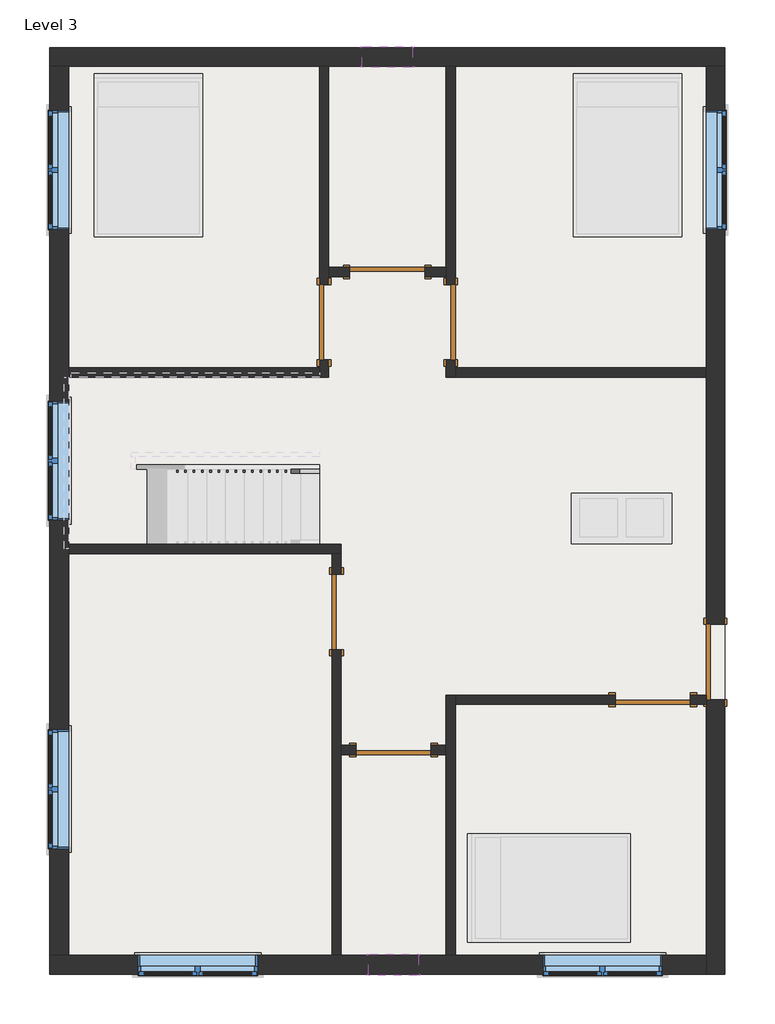
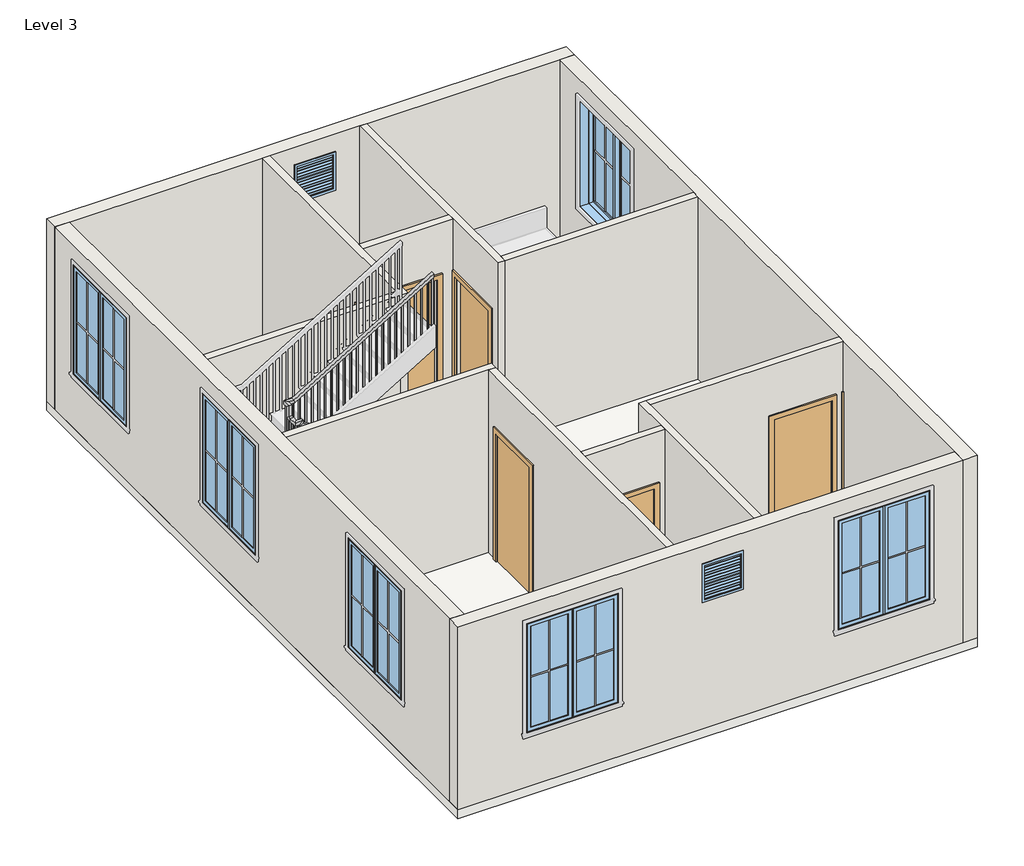
# One storey, part 1 of 2: 14 walls, 8 windows, 7 doors, 1 railing, 1 slab.
"""IFC4 building model written with IfcOpenShell, lengths in millimetres."""

from ifc_helpers import new_model, si_unit, frame, origin, place, context, project, spatial, polyline, outline, extrude, faceted_brep, transform, mapped, element, save
from components import door_305aa2a5, door_e5f9f3c4, door_0ca8825f, window_9ac97e1a, window_f2d8fef0

model = new_model("IFC4")

# Units and contexts
model_context = context("Model", 3, world=origin())
ifc_project = project(units=[si_unit("LENGTHUNIT", "METRE", prefix="MILLI")], contexts=[model_context])

# Site, building, storey
site = spatial("IfcSite", under=ifc_project)
building = spatial("IfcBuilding", under=site)
storey = spatial("IfcBuildingStorey", under=building, Name="Level 3", Elevation=3200.4)

# Doors
placement = place(None, origin())
door_shape = door_305aa2a5(model_context)
element("IfcDoor", 1, ObjectType="Single-Flush : 36\" x 84\"", at=placement, inside=storey, context=model_context, shape_type="MappedRepresentation", body=[
    mapped(door_shape, transform((-2023.6910855, 2116.5303617, 3200.4), x_axis=(0.0, -1.0, 0.0), y_axis=(1.0, 0.0, 0.0), z_axis=(0.0, 0.0, 1.0))),
])
element("IfcDoor", 2, ObjectType="Single-Flush : 36\" x 84\"", at=placement, inside=storey, context=model_context, shape_type="MappedRepresentation", body=[
    mapped(door_shape, transform((-1179.1410855, -3078.1725945, 3200.4), x_axis=(1.0, 0.0, 0.0), y_axis=(0.0, 1.0, 0.0), z_axis=(0.0, 0.0, 1.0))),
])
element("IfcDoor", 3, ObjectType="Single-Flush : 36\" x 84\"", at=placement, inside=storey, context=model_context, shape_type="MappedRepresentation", body=[
    mapped(door_shape, transform((1970.4589145, -2468.1696383, 3200.4), x_axis=(1.0, 0.0, 0.0), y_axis=(0.0, 1.0, 0.0), z_axis=(0.0, 0.0, 1.0))),
])
door_2_shape = door_e5f9f3c4(model_context)
element("IfcDoor", 4, ObjectType="Single-Flush : 36\" x 84\"", at=placement, inside=storey, context=model_context, shape_type="MappedRepresentation", body=[
    mapped(door_2_shape, transform((-486.9910855, 2116.5303617, 3200.4), x_axis=(0.0, -1.0, 0.0), y_axis=(1.0, 0.0, 0.0), z_axis=(0.0, 0.0, 1.0))),
])
element("IfcDoor", 5, ObjectType="Single-Flush : 36\" x 84\"", at=placement, inside=storey, context=model_context, shape_type="MappedRepresentation", body=[
    mapped(door_2_shape, transform((-1871.2910855, -1401.3696383, 3200.4), x_axis=(0.0, 1.0, 0.0), y_axis=(-1.0, 0.0, 0.0), z_axis=(0.0, 0.0, 1.0))),
])
element("IfcDoor", 6, ObjectType="Single-Flush : 36\" x 84\"", at=placement, inside=storey, context=model_context, shape_type="MappedRepresentation", body=[
    mapped(door_2_shape, transform((-1255.3410855, 2726.1303617, 3200.4), x_axis=(1.0, 0.0, 0.0), y_axis=(0.0, 1.0, 0.0), z_axis=(0.0, 0.0, 1.0))),
])
door_3_shape = door_0ca8825f(model_context)
element("IfcDoor", 7, ObjectType="Single-Flush : 36\" x 84\"", at=placement, inside=storey, context=model_context, shape_type="MappedRepresentation", body=[
    mapped(door_3_shape, transform((2732.4589145, -2010.9696383, 3200.4), x_axis=(0.0, 1.0, 0.0), y_axis=(-1.0, 0.0, 0.0), z_axis=(0.0, 0.0, 1.0))),
])

# Railing
element("IfcRailing", 8, ObjectType="Handrail - Rectangular", at=placement, inside=storey, context=model_context, shape_type="SolidModel", body=[
    faceted_brep([(-2080.8410855, 281.3803617, 4253.3454545), (-2080.8410855, 281.3803617, 4193.9439943), (-2080.8410855, 332.1803617, 4193.9439943), (-2080.8410855, 332.1803617, 4253.3454545), (-4290.6410855, 281.3803617, 5592.6181818), (-4341.4410855, 281.3803617, 5564.0046004), (-4341.4410855, 332.1803617, 5564.0046004), (-4290.6410855, 332.1803617, 5592.6181818), (-4290.6410855, 281.3803617, 5638.8), (-4341.4410855, 281.3803617, 5588.0), (-4341.4410855, 332.1803617, 5588.0), (-4290.6410855, 332.1803617, 5638.8), (-4417.6410855, 281.3803617, 5638.8), (-4417.6410855, 281.3803617, 5588.0), (-4366.8410855, 332.1803617, 5588.0), (-4366.8410855, 332.1803617, 5638.8), (-4417.6410855, 408.3803617, 5638.8), (-4417.6410855, 408.3803617, 5588.0), (-4366.8410855, 408.3803617, 5588.0), (-4366.8410855, 408.3803617, 5638.8), (-4417.6410855, 459.1803617, 5638.8), (-4417.6410855, 509.9803617, 5588.0), (-4366.8410855, 509.9803617, 5588.0), (-4366.8410855, 459.1803617, 5638.8), (-4417.6410855, 459.1803617, 5823.5272727), (-4417.6410855, 509.9803617, 5772.7272727), (-4366.8410855, 509.9803617, 5772.7272727), (-4366.8410855, 459.1803617, 5823.5272727), (-4417.6410855, 586.1803617, 5823.5272727), (-4417.6410855, 586.1803617, 5772.7272727), (-4366.8410855, 535.3803617, 5772.7272727), (-4366.8410855, 535.3803617, 5823.5272727), (-4290.6410855, 586.1803617, 5823.5272727), (-4276.4486761, 586.1803617, 5772.7272727), (-4276.4486761, 535.3803617, 5772.7272727), (-4290.6410855, 535.3803617, 5823.5272727), (-2080.8410855, 586.1803617, 7162.8), (-2080.8410855, 535.3803617, 7162.8), (-2080.8410855, 535.3803617, 7103.3985397), (-2080.8410855, 586.1803617, 7103.3985397)], [[[0, 1, 2, 3]], [[1, 0, 4, 5]], [[2, 1, 5, 6]], [[3, 2, 6, 7]], [[0, 3, 7, 4]], [[5, 4, 8, 9]], [[6, 5, 9, 10]], [[7, 6, 10, 11]], [[4, 7, 11, 8]], [[9, 8, 12, 13]], [[10, 9, 13, 14]], [[11, 10, 14, 15]], [[8, 11, 15, 12]], [[13, 12, 16, 17]], [[14, 13, 17, 18]], [[15, 14, 18, 19]], [[12, 15, 19, 16]], [[17, 16, 20, 21]], [[18, 17, 21, 22]], [[19, 18, 22, 23]], [[16, 19, 23, 20]], [[21, 20, 24, 25]], [[22, 21, 25, 26]], [[23, 22, 26, 27]], [[20, 23, 27, 24]], [[25, 24, 28, 29]], [[26, 25, 29, 30]], [[27, 26, 30, 31]], [[24, 27, 31, 28]], [[29, 28, 32, 33]], [[30, 29, 33, 34]], [[31, 30, 34, 35]], [[28, 31, 35, 32]], [[36, 37, 38, 39]], [[33, 32, 36, 39]], [[34, 33, 39, 38]], [[35, 34, 38, 37]], [[32, 35, 37, 36]]]),
    extrude(outline(polyline([(7062.9894488, -2147.5160855), (7051.4439943, -2166.5660855), (6109.8545455, -2166.5660855), (6109.8545455, -2147.5160855), (7062.9894488, -2147.5160855)])), frame((0.0, 551.2553617, 0.0), z_axis=(0.0, 1.0, 0.0), x_axis=(0.0, 0.0, 1.0)), (0.0, 0.0, 1.0), 19.05),
    extrude(outline(polyline([(7001.4136913, -2249.1160855), (6989.8682367, -2268.1660855), (6109.8545455, -2268.1660855), (6109.8545455, -2249.1160855), (7001.4136913, -2249.1160855)])), frame((0.0, 551.2553617, 0.0), z_axis=(0.0, 1.0, 0.0), x_axis=(0.0, 0.0, 1.0)), (0.0, 0.0, 1.0), 19.05),
    extrude(outline(polyline([(6939.8379337, -2350.7160855), (6928.2924791, -2369.7660855), (5971.3090909, -2369.7660855), (5971.3090909, -2350.7160855), (6939.8379337, -2350.7160855)])), frame((0.0, 551.2553617, 0.0), z_axis=(0.0, 1.0, 0.0), x_axis=(0.0, 0.0, 1.0)), (0.0, 0.0, 1.0), 19.05),
    extrude(outline(polyline([(6878.2621761, -2452.3160855), (6866.7167216, -2471.3660855), (5971.3090909, -2471.3660855), (5971.3090909, -2452.3160855), (6878.2621761, -2452.3160855)])), frame((0.0, 551.2553617, 0.0), z_axis=(0.0, 1.0, 0.0), x_axis=(0.0, 0.0, 1.0)), (0.0, 0.0, 1.0), 19.05),
    extrude(outline(polyline([(6816.6864185, -2553.9160855), (6805.140964, -2572.9660855), (5832.7636364, -2572.9660855), (5832.7636364, -2553.9160855), (6816.6864185, -2553.9160855)])), frame((0.0, 551.2553617, 0.0), z_axis=(0.0, 1.0, 0.0), x_axis=(0.0, 0.0, 1.0)), (0.0, 0.0, 1.0), 19.05),
    extrude(outline(polyline([(6755.110661, -2655.5160855), (6743.5652064, -2674.5660855), (5832.7636364, -2674.5660855), (5832.7636364, -2655.5160855), (6755.110661, -2655.5160855)])), frame((0.0, 551.2553617, 0.0), z_axis=(0.0, 1.0, 0.0), x_axis=(0.0, 0.0, 1.0)), (0.0, 0.0, 1.0), 19.05),
    extrude(outline(polyline([(6693.5349034, -2757.1160855), (6681.9894488, -2776.1660855), (5832.7636364, -2776.1660855), (5832.7636364, -2757.1160855), (6693.5349034, -2757.1160855)])), frame((0.0, 551.2553617, 0.0), z_axis=(0.0, 1.0, 0.0), x_axis=(0.0, 0.0, 1.0)), (0.0, 0.0, 1.0), 19.05),
    extrude(outline(polyline([(6631.9591458, -2858.7160855), (6620.4136913, -2877.7660855), (5694.2181818, -2877.7660855), (5694.2181818, -2858.7160855), (6631.9591458, -2858.7160855)])), frame((0.0, 551.2553617, 0.0), z_axis=(0.0, 1.0, 0.0), x_axis=(0.0, 0.0, 1.0)), (0.0, 0.0, 1.0), 19.05),
    extrude(outline(polyline([(6570.3833882, -2960.3160855), (6558.8379337, -2979.3660855), (5694.2181818, -2979.3660855), (5694.2181818, -2960.3160855), (6570.3833882, -2960.3160855)])), frame((0.0, 551.2553617, 0.0), z_axis=(0.0, 1.0, 0.0), x_axis=(0.0, 0.0, 1.0)), (0.0, 0.0, 1.0), 19.05),
    extrude(outline(polyline([(6508.8076307, -3061.9160855), (6497.2621761, -3080.9660855), (5555.6727273, -3080.9660855), (5555.6727273, -3061.9160855), (6508.8076307, -3061.9160855)])), frame((0.0, 551.2553617, 0.0), z_axis=(0.0, 1.0, 0.0), x_axis=(0.0, 0.0, 1.0)), (0.0, 0.0, 1.0), 19.05),
    extrude(outline(polyline([(6447.2318731, -3163.5160855), (6435.6864185, -3182.5660855), (5555.6727273, -3182.5660855), (5555.6727273, -3163.5160855), (6447.2318731, -3163.5160855)])), frame((0.0, 551.2553617, 0.0), z_axis=(0.0, 1.0, 0.0), x_axis=(0.0, 0.0, 1.0)), (0.0, 0.0, 1.0), 19.05),
    extrude(outline(polyline([(6385.6561155, -3265.1160855), (6374.110661, -3284.1660855), (5417.1272727, -3284.1660855), (5417.1272727, -3265.1160855), (6385.6561155, -3265.1160855)])), frame((0.0, 551.2553617, 0.0), z_axis=(0.0, 1.0, 0.0), x_axis=(0.0, 0.0, 1.0)), (0.0, 0.0, 1.0), 19.05),
    extrude(outline(polyline([(6324.0803579, -3366.7160855), (6312.5349034, -3385.7660855), (5417.1272727, -3385.7660855), (5417.1272727, -3366.7160855), (6324.0803579, -3366.7160855)])), frame((0.0, 551.2553617, 0.0), z_axis=(0.0, 1.0, 0.0), x_axis=(0.0, 0.0, 1.0)), (0.0, 0.0, 1.0), 19.05),
    extrude(outline(polyline([(6262.5046004, -3468.3160855), (6250.9591458, -3487.3660855), (5278.5818182, -3487.3660855), (5278.5818182, -3468.3160855), (6262.5046004, -3468.3160855)])), frame((0.0, 551.2553617, 0.0), z_axis=(0.0, 1.0, 0.0), x_axis=(0.0, 0.0, 1.0)), (0.0, 0.0, 1.0), 19.05),
    extrude(outline(polyline([(6200.9288428, -3569.9160855), (6189.3833882, -3588.9660855), (5278.5818182, -3588.9660855), (5278.5818182, -3569.9160855), (6200.9288428, -3569.9160855)])), frame((0.0, 551.2553617, 0.0), z_axis=(0.0, 1.0, 0.0), x_axis=(0.0, 0.0, 1.0)), (0.0, 0.0, 1.0), 19.05),
    extrude(outline(polyline([(6139.3530852, -3671.5160855), (6127.8076307, -3690.5660855), (5278.5818182, -3690.5660855), (5278.5818182, -3671.5160855), (6139.3530852, -3671.5160855)])), frame((0.0, 551.2553617, 0.0), z_axis=(0.0, 1.0, 0.0), x_axis=(0.0, 0.0, 1.0)), (0.0, 0.0, 1.0), 19.05),
    extrude(outline(polyline([(6077.7773276, -3773.1160855), (6066.2318731, -3792.1660855), (5140.0363636, -3792.1660855), (5140.0363636, -3773.1160855), (6077.7773276, -3773.1160855)])), frame((0.0, 551.2553617, 0.0), z_axis=(0.0, 1.0, 0.0), x_axis=(0.0, 0.0, 1.0)), (0.0, 0.0, 1.0), 19.05),
    extrude(outline(polyline([(6016.20157, -3874.7160855), (6004.6561155, -3893.7660855), (5140.0363636, -3893.7660855), (5140.0363636, -3874.7160855), (6016.20157, -3874.7160855)])), frame((0.0, 551.2553617, 0.0), z_axis=(0.0, 1.0, 0.0), x_axis=(0.0, 0.0, 1.0)), (0.0, 0.0, 1.0), 19.05),
    extrude(outline(polyline([(5954.6258125, -3976.3160855), (5943.0803579, -3995.3660855), (5001.4909091, -3995.3660855), (5001.4909091, -3976.3160855), (5954.6258125, -3976.3160855)])), frame((0.0, 551.2553617, 0.0), z_axis=(0.0, 1.0, 0.0), x_axis=(0.0, 0.0, 1.0)), (0.0, 0.0, 1.0), 19.05),
    extrude(outline(polyline([(5893.0500549, -4077.9160855), (5881.5046004, -4096.9660855), (5001.4909091, -4096.9660855), (5001.4909091, -4077.9160855), (5893.0500549, -4077.9160855)])), frame((0.0, 551.2553617, 0.0), z_axis=(0.0, 1.0, 0.0), x_axis=(0.0, 0.0, 1.0)), (0.0, 0.0, 1.0), 19.05),
    extrude(outline(polyline([(5831.4742973, -4179.5160855), (5819.9288428, -4198.5660855), (4862.9454545, -4198.5660855), (4862.9454545, -4179.5160855), (5831.4742973, -4179.5160855)])), frame((0.0, 551.2553617, 0.0), z_axis=(0.0, 1.0, 0.0), x_axis=(0.0, 0.0, 1.0)), (0.0, 0.0, 1.0), 19.05),
    extrude(outline(polyline([(5769.8985397, -4281.1160855), (5758.3530852, -4300.1660855), (4862.9454545, -4300.1660855), (4862.9454545, -4281.1160855), (5769.8985397, -4281.1160855)])), frame((0.0, 551.2553617, 0.0), z_axis=(0.0, 1.0, 0.0), x_axis=(0.0, 0.0, 1.0)), (0.0, 0.0, 1.0), 19.05),
    extrude(outline(polyline([(-4382.7160855, 500.4553617), (-4401.7660855, 500.4553617), (-4401.7660855, 519.5053617), (-4382.7160855, 519.5053617), (-4382.7160855, 500.4553617)])), frame((0.0, 0.0, 4724.4), z_axis=(0.0, 0.0, 1.0), x_axis=(1.0, 0.0, 0.0)), (0.0, 0.0, 1.0), 1048.3272727),
    extrude(outline(polyline([(-4382.7160855, 398.8553617), (-4401.7660855, 398.8553617), (-4401.7660855, 417.9053617), (-4382.7160855, 417.9053617), (-4382.7160855, 398.8553617)])), frame((0.0, 0.0, 4724.4), z_axis=(0.0, 0.0, 1.0), x_axis=(1.0, 0.0, 0.0)), (0.0, 0.0, 1.0), 863.6),
    extrude(outline(polyline([(-4306.5160855, 316.3053617), (-4306.5160855, 297.2553617), (-4325.5660855, 297.2553617), (-4325.5660855, 316.3053617), (-4306.5160855, 316.3053617)])), frame((0.0, 0.0, 4585.8545455), z_axis=(0.0, 0.0, 1.0), x_axis=(1.0, 0.0, 0.0)), (0.0, 0.0, 1.0), 1002.1454545),
    extrude(outline(polyline([(5481.2621761, -4204.9160855), (5492.8076307, -4223.9660855), (4585.8545455, -4223.9660855), (4585.8545455, -4204.9160855), (5481.2621761, -4204.9160855)])), frame((0.0, 297.2553617, 0.0), z_axis=(0.0, 1.0, 0.0), x_axis=(0.0, 0.0, 1.0)), (0.0, 0.0, 1.0), 19.05),
    extrude(outline(polyline([(5419.6864185, -4103.3160855), (5431.2318731, -4122.3660855), (4447.3090909, -4122.3660855), (4447.3090909, -4103.3160855), (5419.6864185, -4103.3160855)])), frame((0.0, 297.2553617, 0.0), z_axis=(0.0, 1.0, 0.0), x_axis=(0.0, 0.0, 1.0)), (0.0, 0.0, 1.0), 19.05),
    extrude(outline(polyline([(5358.110661, -4001.7160855), (5369.6561155, -4020.7660855), (4447.3090909, -4020.7660855), (4447.3090909, -4001.7160855), (5358.110661, -4001.7160855)])), frame((0.0, 297.2553617, 0.0), z_axis=(0.0, 1.0, 0.0), x_axis=(0.0, 0.0, 1.0)), (0.0, 0.0, 1.0), 19.05),
    extrude(outline(polyline([(5296.5349034, -3900.1160855), (5308.0803579, -3919.1660855), (4447.3090909, -3919.1660855), (4447.3090909, -3900.1160855), (5296.5349034, -3900.1160855)])), frame((0.0, 297.2553617, 0.0), z_axis=(0.0, 1.0, 0.0), x_axis=(0.0, 0.0, 1.0)), (0.0, 0.0, 1.0), 19.05),
    extrude(outline(polyline([(5234.9591458, -3798.5160855), (5246.5046004, -3817.5660855), (4308.7636364, -3817.5660855), (4308.7636364, -3798.5160855), (5234.9591458, -3798.5160855)])), frame((0.0, 297.2553617, 0.0), z_axis=(0.0, 1.0, 0.0), x_axis=(0.0, 0.0, 1.0)), (0.0, 0.0, 1.0), 19.05),
    extrude(outline(polyline([(5173.3833882, -3696.9160855), (5184.9288428, -3715.9660855), (4308.7636364, -3715.9660855), (4308.7636364, -3696.9160855), (5173.3833882, -3696.9160855)])), frame((0.0, 297.2553617, 0.0), z_axis=(0.0, 1.0, 0.0), x_axis=(0.0, 0.0, 1.0)), (0.0, 0.0, 1.0), 19.05),
    extrude(outline(polyline([(5111.8076307, -3595.3160855), (5123.3530852, -3614.3660855), (4170.2181818, -3614.3660855), (4170.2181818, -3595.3160855), (5111.8076307, -3595.3160855)])), frame((0.0, 297.2553617, 0.0), z_axis=(0.0, 1.0, 0.0), x_axis=(0.0, 0.0, 1.0)), (0.0, 0.0, 1.0), 19.05),
    extrude(outline(polyline([(5050.2318731, -3493.7160855), (5061.7773276, -3512.7660855), (4170.2181818, -3512.7660855), (4170.2181818, -3493.7160855), (5050.2318731, -3493.7160855)])), frame((0.0, 297.2553617, 0.0), z_axis=(0.0, 1.0, 0.0), x_axis=(0.0, 0.0, 1.0)), (0.0, 0.0, 1.0), 19.05),
    extrude(outline(polyline([(4988.6561155, -3392.1160855), (5000.20157, -3411.1660855), (4031.6727273, -3411.1660855), (4031.6727273, -3392.1160855), (4988.6561155, -3392.1160855)])), frame((0.0, 297.2553617, 0.0), z_axis=(0.0, 1.0, 0.0), x_axis=(0.0, 0.0, 1.0)), (0.0, 0.0, 1.0), 19.05),
    extrude(outline(polyline([(4927.0803579, -3290.5160855), (4938.6258125, -3309.5660855), (4031.6727273, -3309.5660855), (4031.6727273, -3290.5160855), (4927.0803579, -3290.5160855)])), frame((0.0, 297.2553617, 0.0), z_axis=(0.0, 1.0, 0.0), x_axis=(0.0, 0.0, 1.0)), (0.0, 0.0, 1.0), 19.05),
    extrude(outline(polyline([(4865.5046004, -3188.9160855), (4877.0500549, -3207.9660855), (3893.1272727, -3207.9660855), (3893.1272727, -3188.9160855), (4865.5046004, -3188.9160855)])), frame((0.0, 297.2553617, 0.0), z_axis=(0.0, 1.0, 0.0), x_axis=(0.0, 0.0, 1.0)), (0.0, 0.0, 1.0), 19.05),
    extrude(outline(polyline([(4803.9288428, -3087.3160855), (4815.4742973, -3106.3660855), (3893.1272727, -3106.3660855), (3893.1272727, -3087.3160855), (4803.9288428, -3087.3160855)])), frame((0.0, 297.2553617, 0.0), z_axis=(0.0, 1.0, 0.0), x_axis=(0.0, 0.0, 1.0)), (0.0, 0.0, 1.0), 19.05),
    extrude(outline(polyline([(4742.3530852, -2985.7160855), (4753.8985397, -3004.7660855), (3893.1272727, -3004.7660855), (3893.1272727, -2985.7160855), (4742.3530852, -2985.7160855)])), frame((0.0, 297.2553617, 0.0), z_axis=(0.0, 1.0, 0.0), x_axis=(0.0, 0.0, 1.0)), (0.0, 0.0, 1.0), 19.05),
    extrude(outline(polyline([(4680.7773276, -2884.1160855), (4692.3227822, -2903.1660855), (3754.5818182, -2903.1660855), (3754.5818182, -2884.1160855), (4680.7773276, -2884.1160855)])), frame((0.0, 297.2553617, 0.0), z_axis=(0.0, 1.0, 0.0), x_axis=(0.0, 0.0, 1.0)), (0.0, 0.0, 1.0), 19.05),
    extrude(outline(polyline([(4619.20157, -2782.5160855), (4630.7470246, -2801.5660855), (3754.5818182, -2801.5660855), (3754.5818182, -2782.5160855), (4619.20157, -2782.5160855)])), frame((0.0, 297.2553617, 0.0), z_axis=(0.0, 1.0, 0.0), x_axis=(0.0, 0.0, 1.0)), (0.0, 0.0, 1.0), 19.05),
    extrude(outline(polyline([(4557.6258125, -2680.9160855), (4569.171267, -2699.9660855), (3616.0363636, -2699.9660855), (3616.0363636, -2680.9160855), (4557.6258125, -2680.9160855)])), frame((0.0, 297.2553617, 0.0), z_axis=(0.0, 1.0, 0.0), x_axis=(0.0, 0.0, 1.0)), (0.0, 0.0, 1.0), 19.05),
    extrude(outline(polyline([(4496.0500549, -2579.3160855), (4507.5955094, -2598.3660855), (3616.0363636, -2598.3660855), (3616.0363636, -2579.3160855), (4496.0500549, -2579.3160855)])), frame((0.0, 297.2553617, 0.0), z_axis=(0.0, 1.0, 0.0), x_axis=(0.0, 0.0, 1.0)), (0.0, 0.0, 1.0), 19.05),
    extrude(outline(polyline([(4434.4742973, -2477.7160855), (4446.0197519, -2496.7660855), (3477.4909091, -2496.7660855), (3477.4909091, -2477.7160855), (4434.4742973, -2477.7160855)])), frame((0.0, 297.2553617, 0.0), z_axis=(0.0, 1.0, 0.0), x_axis=(0.0, 0.0, 1.0)), (0.0, 0.0, 1.0), 19.05),
    extrude(outline(polyline([(4372.8985397, -2376.1160855), (4384.4439943, -2395.1660855), (3477.4909091, -2395.1660855), (3477.4909091, -2376.1160855), (4372.8985397, -2376.1160855)])), frame((0.0, 297.2553617, 0.0), z_axis=(0.0, 1.0, 0.0), x_axis=(0.0, 0.0, 1.0)), (0.0, 0.0, 1.0), 19.05),
    extrude(outline(polyline([(4311.3227822, -2274.5160855), (4322.8682367, -2293.5660855), (3338.9454545, -2293.5660855), (3338.9454545, -2274.5160855), (4311.3227822, -2274.5160855)])), frame((0.0, 297.2553617, 0.0), z_axis=(0.0, 1.0, 0.0), x_axis=(0.0, 0.0, 1.0)), (0.0, 0.0, 1.0), 19.05),
    extrude(outline(polyline([(4249.7470246, -2172.9160855), (4261.2924791, -2191.9660855), (3338.9454545, -2191.9660855), (3338.9454545, -2172.9160855), (4249.7470246, -2172.9160855)])), frame((0.0, 297.2553617, 0.0), z_axis=(0.0, 1.0, 0.0), x_axis=(0.0, 0.0, 1.0)), (0.0, 0.0, 1.0), 19.05),
    extrude(outline(polyline([(-4382.7160855, 551.2553617), (-4401.7660855, 551.2553617), (-4401.7660855, 570.3053617), (-4382.7160855, 570.3053617), (-4382.7160855, 551.2553617)])), frame((0.0, 0.0, 4724.4), z_axis=(0.0, 0.0, 1.0), x_axis=(1.0, 0.0, 0.0)), (0.0, 0.0, 1.0), 1048.3272727),
    extrude(outline(polyline([(-4382.7160855, 316.3053617), (-4382.7160855, 297.2553617), (-4401.7660855, 297.2553617), (-4401.7660855, 316.3053617), (-4382.7160855, 316.3053617)])), frame((0.0, 0.0, 4724.4), z_axis=(0.0, 0.0, 1.0), x_axis=(1.0, 0.0, 0.0)), (0.0, 0.0, 1.0), 863.6),
    extrude(outline(polyline([(7103.3985397, -2080.8410855), (7091.8530852, -2099.8910855), (6109.8545455, -2099.8910855), (6109.8545455, -2080.8410855), (7103.3985397, -2080.8410855)])), frame((0.0, 551.2553617, 0.0), z_axis=(0.0, 1.0, 0.0), x_axis=(0.0, 0.0, 1.0)), (0.0, 0.0, 1.0), 19.05),
    extrude(outline(polyline([(4193.9439943, -2080.8410855), (4205.4894488, -2099.8910855), (3338.9454545, -2099.8910855), (3338.9454545, -2080.8410855), (4193.9439943, -2080.8410855)])), frame((0.0, 297.2553617, 0.0), z_axis=(0.0, 1.0, 0.0), x_axis=(0.0, 0.0, 1.0)), (0.0, 0.0, 1.0), 19.05),
])

# Slab
element("IfcSlab", 9, ObjectType="FLOOR 6\"", at=placement, inside=storey, context=model_context, shape_type="SweptSolid", body=[
    extrude(outline(polyline([(2846.7589145, 5450.2803617), (2846.7589145, -5801.9196383), (-5357.4410855, -5801.9196383), (-5357.4410855, 5450.2803617), (2846.7589145, 5450.2803617)])), frame((0.0, 0.0, 3048.0), z_axis=(0.0, 0.0, 1.0), x_axis=(1.0, 0.0, 0.0)), (0.0, 0.0, 1.0), 152.4),
])

# Walls
element("IfcWall", 10, ObjectType="WALL 4.5\"", at=placement, inside=storey, context=model_context, shape_type="Brep", body=[
    faceted_brep([(-2080.8410855, 1659.3303617, 5334.0), (-2080.8410855, 1659.3303617, 3200.4), (-2080.8410855, 1564.0803617, 3200.4), (-2080.8410855, 1449.7803617, 3200.4), (-2080.8410855, 1449.7803617, 6248.4), (-2080.8410855, 1564.0803617, 6248.4), (-2080.8410855, 5221.6803617, 6248.4), (-2080.8410855, 5221.6803617, 3200.4), (-2080.8410855, 2573.7303617, 3200.4), (-2080.8410855, 2573.7303617, 5334.0), (-1966.5410855, 1449.7803617, 3200.4), (-1966.5410855, 1659.3303617, 3200.4), (-1966.5410855, 1659.3303617, 5334.0), (-1966.5410855, 2573.7303617, 5334.0), (-1966.5410855, 2573.7303617, 3200.4), (-1966.5410855, 2668.9803617, 3200.4), (-1966.5410855, 2783.2803617, 3200.4), (-1966.5410855, 5221.6803617, 3200.4), (-1966.5410855, 5221.6803617, 6248.4), (-1966.5410855, 2783.2803617, 6248.4), (-1966.5410855, 2668.9803617, 6248.4), (-1966.5410855, 1449.7803617, 6248.4)], [[[0, 1, 2, 3, 4, 5, 6, 7, 8, 9]], [[10, 11, 12, 13, 14, 15, 16, 17, 18, 19, 20, 21]], [[8, 7, 17, 16, 15, 14]], [[3, 2, 1, 11, 10]], [[7, 6, 18, 17]], [[4, 3, 10, 21]], [[12, 11, 1, 0]], [[13, 12, 0, 9]], [[14, 13, 9, 8]], [[6, 5, 4, 21, 20, 19, 18]]]),
])
element("IfcWall", 11, ObjectType="WALL 4.5\"", at=placement, inside=storey, context=model_context, shape_type="SweptSolid", body=[
    extrude(outline(polyline([(-5128.8410855, 1564.0803617), (-2080.8410855, 1564.0803617), (-2080.8410855, 1449.7803617), (-5128.8410855, 1449.7803617), (-5128.8410855, 1564.0803617)])), frame((0.0, 0.0, 3200.4), z_axis=(0.0, 0.0, 1.0), x_axis=(1.0, 0.0, 0.0)), (0.0, 0.0, 1.0), 3048.0),
])
element("IfcWall", 12, ObjectType="WALL 4.5\"", at=placement, inside=storey, context=model_context, shape_type="Brep", body=[
    faceted_brep([(-544.1410855, 1659.3303617, 5334.0), (-544.1410855, 1659.3303617, 3200.4), (-544.1410855, 1449.7803617, 3200.4), (-544.1410855, 1449.7803617, 6248.4), (-544.1410855, 2668.9803617, 6248.4), (-544.1410855, 2783.2803617, 6248.4), (-544.1410855, 5221.6803617, 6248.4), (-544.1410855, 5221.6803617, 3200.4), (-544.1410855, 2783.2803617, 3200.4), (-544.1410855, 2668.9803617, 3200.4), (-544.1410855, 2573.7303617, 3200.4), (-544.1410855, 2573.7303617, 5334.0), (-429.8410855, 1449.7803617, 3200.4), (-429.8410855, 1564.0803617, 3200.4), (-429.8410855, 1659.3303617, 3200.4), (-429.8410855, 1659.3303617, 5334.0), (-429.8410855, 2573.7303617, 5334.0), (-429.8410855, 2573.7303617, 3200.4), (-429.8410855, 5221.6803617, 3200.4), (-429.8410855, 5221.6803617, 6248.4), (-429.8410855, 1564.0803617, 6248.4), (-429.8410855, 1449.7803617, 6248.4)], [[[0, 1, 2, 3, 4, 5, 6, 7, 8, 9, 10, 11]], [[12, 13, 14, 15, 16, 17, 18, 19, 20, 21]], [[2, 1, 14, 13, 12]], [[10, 9, 8, 7, 18, 17]], [[7, 6, 19, 18]], [[3, 2, 12, 21]], [[15, 14, 1, 0]], [[16, 15, 0, 11]], [[17, 16, 11, 10]], [[6, 5, 4, 3, 21, 20, 19]]]),
])
element("IfcWall", 13, ObjectType="WALL 4.5\"", at=placement, inside=storey, context=model_context, shape_type="SweptSolid", body=[
    extrude(outline(polyline([(2618.1589145, 1449.7803617), (-429.8410855, 1449.7803617), (-429.8410855, 1564.0803617), (2618.1589145, 1564.0803617), (2618.1589145, 1449.7803617)])), frame((0.0, 0.0, 3200.4), z_axis=(0.0, 0.0, 1.0), x_axis=(1.0, 0.0, 0.0)), (0.0, 0.0, 1.0), 3048.0),
])
element("IfcWall", 14, ObjectType="WALL 4.5\"", at=placement, inside=storey, context=model_context, shape_type="Brep", body=[
    faceted_brep([(-5128.8410855, -696.5196383, 3200.4), (-1928.4410855, -696.5196383, 3200.4), (-1814.1410855, -696.5196383, 3200.4), (-1814.1410855, -696.5196383, 6248.4), (-1928.4410855, -696.5196383, 6248.4), (-5128.8410855, -696.5196383, 6248.4), (-5128.8410855, -582.2196383, 3200.4), (-5128.8410855, -582.2196383, 6248.4), (-1814.1410855, -582.2196383, 6248.4), (-1814.1410855, -582.2196383, 3200.4)], [[[0, 1, 2, 3, 4, 5]], [[6, 7, 8, 9]], [[2, 1, 0, 6, 9]], [[0, 5, 7, 6]], [[3, 2, 9, 8]], [[5, 4, 3, 8, 7]]]),
])
element("IfcWall", 15, ObjectType="WALL 4.5\"", at=placement, inside=storey, context=model_context, shape_type="Brep", body=[
    faceted_brep([(-1814.1410855, -944.1696383, 5334.0), (-1814.1410855, -944.1696383, 3200.4), (-1814.1410855, -696.5196383, 3200.4), (-1814.1410855, -696.5196383, 6248.4), (-1814.1410855, -3021.0225945, 6248.4), (-1814.1410855, -3135.3225945, 6248.4), (-1814.1410855, -5573.3196383, 6248.4), (-1814.1410855, -5573.3196383, 3200.4), (-1814.1410855, -3135.3225945, 3200.4), (-1814.1410855, -3021.0225945, 3200.4), (-1814.1410855, -1858.5696383, 3200.4), (-1814.1410855, -1858.5696383, 5334.0), (-1928.4410855, -696.5196383, 3200.4), (-1928.4410855, -944.1696383, 3200.4), (-1928.4410855, -944.1696383, 5334.0), (-1928.4410855, -1858.5696383, 5334.0), (-1928.4410855, -1858.5696383, 3200.4), (-1928.4410855, -5573.3196383, 3200.4), (-1928.4410855, -5573.3196383, 6248.4), (-1928.4410855, -696.5196383, 6248.4)], [[[0, 1, 2, 3, 4, 5, 6, 7, 8, 9, 10, 11]], [[12, 13, 14, 15, 16, 17, 18, 19]], [[2, 1, 13, 12]], [[10, 9, 8, 7, 17, 16]], [[3, 2, 12, 19]], [[7, 6, 18, 17]], [[14, 13, 1, 0]], [[15, 14, 0, 11]], [[16, 15, 11, 10]], [[6, 5, 4, 3, 19, 18]]]),
])
element("IfcWall", 16, ObjectType="WALL 4.5\"", at=placement, inside=storey, context=model_context, shape_type="SweptSolid", body=[
    extrude(outline(polyline([(5334.0, -721.9410855), (3200.4, -721.9410855), (3200.4, -544.1410855), (6248.4, -544.1410855), (6248.4, -1814.1410855), (3200.4, -1814.1410855), (3200.4, -1636.3410855), (5334.0, -1636.3410855), (5334.0, -721.9410855)])), frame((0.0, -3135.3225945, 0.0), z_axis=(0.0, 1.0, 0.0), x_axis=(0.0, 0.0, 1.0)), (0.0, 0.0, 1.0), 114.3),
])
element("IfcWall", 17, ObjectType="WALL 4.5\"", at=placement, inside=storey, context=model_context, shape_type="Brep", body=[
    faceted_brep([(-544.1410855, -2411.0196383, 3200.4), (-544.1410855, -3021.0225945, 3200.4), (-544.1410855, -3135.3225945, 3200.4), (-544.1410855, -5573.3196383, 3200.4), (-544.1410855, -5573.3196383, 6248.4), (-544.1410855, -3135.3225945, 6248.4), (-544.1410855, -3021.0225945, 6248.4), (-544.1410855, -2411.0196383, 6248.4), (-429.8410855, -2411.0196383, 3200.4), (-429.8410855, -2411.0196383, 6248.4), (-429.8410855, -2525.3196383, 6248.4), (-429.8410855, -5573.3196383, 6248.4), (-429.8410855, -5573.3196383, 3200.4), (-429.8410855, -2525.3196383, 3200.4)], [[[0, 1, 2, 3, 4, 5, 6, 7]], [[8, 9, 10, 11, 12, 13]], [[3, 2, 1, 0, 8, 13, 12]], [[4, 3, 12, 11]], [[0, 7, 9, 8]], [[7, 6, 5, 4, 11, 10, 9]]]),
])
element("IfcWall", 18, ObjectType="WALL 4.5\"", at=placement, inside=storey, context=model_context, shape_type="Brep", body=[
    faceted_brep([(2427.6589145, -2525.3196383, 5334.0), (2427.6589145, -2525.3196383, 3200.4), (2618.1589145, -2525.3196383, 3200.4), (2618.1589145, -2525.3196383, 6248.4), (-429.8410855, -2525.3196383, 6248.4), (-429.8410855, -2525.3196383, 3200.4), (1513.2589145, -2525.3196383, 3200.4), (1513.2589145, -2525.3196383, 5334.0), (2618.1589145, -2411.0196383, 3200.4), (2427.6589145, -2411.0196383, 3200.4), (2427.6589145, -2411.0196383, 5334.0), (1513.2589145, -2411.0196383, 5334.0), (1513.2589145, -2411.0196383, 3200.4), (-429.8410855, -2411.0196383, 3200.4), (-429.8410855, -2411.0196383, 6248.4), (2618.1589145, -2411.0196383, 6248.4), (2618.1589145, -2468.1696383, 3200.4)], [[[0, 1, 2, 3, 4, 5, 6, 7]], [[8, 9, 10, 11, 12, 13, 14, 15]], [[6, 5, 13, 12]], [[2, 1, 9, 8, 16]], [[5, 4, 14, 13]], [[3, 2, 16, 8, 15]], [[10, 9, 1, 0]], [[11, 10, 0, 7]], [[12, 11, 7, 6]], [[4, 3, 15, 14]]]),
])
element("IfcWall", 19, ObjectType="WALL 4.5\"", at=placement, inside=storey, context=model_context, shape_type="SweptSolid", body=[
    extrude(outline(polyline([(5334.0, -798.1410855), (3200.4, -798.1410855), (3200.4, -544.1410855), (6248.4, -544.1410855), (6248.4, -1966.5410855), (3200.4, -1966.5410855), (3200.4, -1712.5410855), (5334.0, -1712.5410855), (5334.0, -798.1410855)])), frame((0.0, 2668.9803617, 0.0), z_axis=(0.0, 1.0, 0.0), x_axis=(0.0, 0.0, 1.0)), (0.0, 0.0, 1.0), 114.3),
])
element("IfcWall", 20, ObjectType="WALL 9\"", at=placement, inside=storey, context=model_context, shape_type="Brep", body=[
    faceted_brep([(-5357.4410855, 5221.6803617, 3200.4), (-5128.8410855, 5221.6803617, 3200.4), (-2080.8410855, 5221.6803617, 3200.4), (-1966.5410855, 5221.6803617, 3200.4), (-544.1410855, 5221.6803617, 3200.4), (-429.8410855, 5221.6803617, 3200.4), (2618.1589145, 5221.6803617, 3200.4), (2846.7589145, 5221.6803617, 3200.4), (2846.7589145, 5221.6803617, 6248.4), (2618.1589145, 5221.6803617, 6248.4), (-429.8410855, 5221.6803617, 6248.4), (-544.1410855, 5221.6803617, 6248.4), (-1966.5410855, 5221.6803617, 6248.4), (-2080.8410855, 5221.6803617, 6248.4), (-5128.8410855, 5221.6803617, 6248.4), (-5357.4410855, 5221.6803617, 6248.4), (-950.5410855, 5221.6803617, 5943.6), (-950.5410855, 5221.6803617, 5334.0), (-1560.1410855, 5221.6803617, 5334.0), (-1560.1410855, 5221.6803617, 5943.6), (-5357.4410855, 5450.2803617, 3200.4), (-5357.4410855, 5450.2803617, 6248.4), (2846.7589145, 5450.2803617, 6248.4), (2846.7589145, 5450.2803617, 3200.4), (-950.5410855, 5450.2803617, 5943.6), (-1560.1410855, 5450.2803617, 5943.6), (-1560.1410855, 5450.2803617, 5334.0), (-950.5410855, 5450.2803617, 5334.0)], [[[0, 1, 2, 3, 4, 5, 6, 7, 8, 9, 10, 11, 12, 13, 14, 15], [16, 17, 18, 19]], [[20, 21, 22, 23], [24, 25, 26, 27]], [[7, 6, 5, 4, 3, 2, 1, 0, 20, 23]], [[8, 7, 23, 22]], [[0, 15, 21, 20]], [[17, 16, 24, 27]], [[18, 17, 27, 26]], [[19, 18, 26, 25]], [[16, 19, 25, 24]], [[15, 14, 13, 12, 11, 10, 9, 8, 22, 21]]]),
])
element("IfcWall", 21, ObjectType="WALL 9\"", at=placement, inside=storey, context=model_context, shape_type="Brep", body=[
    faceted_brep([(2618.1589145, 5221.6803617, 3200.4), (2618.1589145, 1564.0803617, 3200.4), (2618.1589145, 1449.7803617, 3200.4), (2618.1589145, -1553.7696383, 3200.4), (2618.1589145, -1553.7696383, 5334.0), (2618.1589145, -2468.1696383, 5334.0), (2618.1589145, -2468.1696383, 3200.4), (2618.1589145, -2525.3196383, 3200.4), (2618.1589145, -5573.3196383, 3200.4), (2618.1589145, -5801.9196383, 3200.4), (2618.1589145, -5801.9196383, 6248.4), (2618.1589145, -5573.3196383, 6248.4), (2618.1589145, -2525.3196383, 6248.4), (2618.1589145, -2411.0196383, 6248.4), (2618.1589145, 1449.7803617, 6248.4), (2618.1589145, 1564.0803617, 6248.4), (2618.1589145, 5221.6803617, 6248.4), (2618.1589145, 3240.4803617, 5943.6), (2618.1589145, 3240.4803617, 4114.8), (2618.1589145, 4688.2803617, 4114.8), (2618.1589145, 4688.2803617, 5943.6), (2846.7589145, -1553.7696383, 5334.0), (2846.7589145, -1553.7696383, 3200.4), (2846.7589145, 5221.6803617, 3200.4), (2846.7589145, 5221.6803617, 6248.4), (2846.7589145, -5801.9196383, 6248.4), (2846.7589145, -5801.9196383, 3200.4), (2846.7589145, -2468.1696383, 3200.4), (2846.7589145, -2468.1696383, 5334.0), (2846.7589145, 3240.4803617, 5943.6), (2846.7589145, 4688.2803617, 5943.6), (2846.7589145, 4688.2803617, 4114.8), (2846.7589145, 3240.4803617, 4114.8)], [[[0, 1, 2, 3, 4, 5, 6, 7, 8, 9, 10, 11, 12, 13, 14, 15, 16], [17, 18, 19, 20]], [[21, 22, 23, 24, 25, 26, 27, 28], [29, 30, 31, 32]], [[27, 26, 9, 8, 7, 6]], [[23, 22, 3, 2, 1, 0]], [[0, 16, 24, 23]], [[10, 9, 26, 25]], [[18, 17, 29, 32]], [[19, 18, 32, 31]], [[20, 19, 31, 30]], [[17, 20, 30, 29]], [[4, 3, 22, 21]], [[5, 4, 21, 28]], [[6, 5, 28, 27]], [[16, 15, 14, 13, 12, 11, 10, 25, 24]]]),
])
element("IfcWall", 22, ObjectType="WALL 9\"", at=placement, inside=storey, context=model_context, shape_type="Brep", body=[
    faceted_brep([(2618.1589145, -5573.3196383, 3200.4), (-429.8410855, -5573.3196383, 3200.4), (-544.1410855, -5573.3196383, 3200.4), (-1814.1410855, -5573.3196383, 3200.4), (-1928.4410855, -5573.3196383, 3200.4), (-5128.8410855, -5573.3196383, 3200.4), (-5357.4410855, -5573.3196383, 3200.4), (-5357.4410855, -5573.3196383, 6248.4), (-5128.8410855, -5573.3196383, 6248.4), (-1928.4410855, -5573.3196383, 6248.4), (-1814.1410855, -5573.3196383, 6248.4), (-544.1410855, -5573.3196383, 6248.4), (-429.8410855, -5573.3196383, 6248.4), (2618.1589145, -5573.3196383, 6248.4), (-4281.1160855, -5573.3196383, 5943.6), (-4281.1160855, -5573.3196383, 4114.8), (-2833.3160855, -5573.3196383, 4114.8), (-2833.3160855, -5573.3196383, 5943.6), (636.9589145, -5573.3196383, 5943.6), (636.9589145, -5573.3196383, 4114.8), (2084.7589145, -5573.3196383, 4114.8), (2084.7589145, -5573.3196383, 5943.6), (-874.3410855, -5573.3196383, 5943.6), (-1483.9410855, -5573.3196383, 5943.6), (-1483.9410855, -5573.3196383, 5334.0), (-874.3410855, -5573.3196383, 5334.0), (2618.1589145, -5801.9196383, 3200.4), (2618.1589145, -5801.9196383, 6248.4), (-5357.4410855, -5801.9196383, 6248.4), (-5357.4410855, -5801.9196383, 3200.4), (-4281.1160855, -5801.9196383, 5943.6), (-2833.3160855, -5801.9196383, 5943.6), (-2833.3160855, -5801.9196383, 4114.8), (-4281.1160855, -5801.9196383, 4114.8), (636.9589145, -5801.9196383, 5943.6), (2084.7589145, -5801.9196383, 5943.6), (2084.7589145, -5801.9196383, 4114.8), (636.9589145, -5801.9196383, 4114.8), (-874.3410855, -5801.9196383, 5943.6), (-874.3410855, -5801.9196383, 5334.0), (-1483.9410855, -5801.9196383, 5334.0), (-1483.9410855, -5801.9196383, 5943.6)], [[[0, 1, 2, 3, 4, 5, 6, 7, 8, 9, 10, 11, 12, 13], [14, 15, 16, 17], [18, 19, 20, 21], [22, 23, 24, 25]], [[26, 27, 28, 29], [30, 31, 32, 33], [34, 35, 36, 37], [38, 39, 40, 41]], [[6, 5, 4, 3, 2, 1, 0, 26, 29]], [[0, 13, 27, 26]], [[7, 6, 29, 28]], [[15, 14, 30, 33]], [[16, 15, 33, 32]], [[17, 16, 32, 31]], [[14, 17, 31, 30]], [[19, 18, 34, 37]], [[20, 19, 37, 36]], [[21, 20, 36, 35]], [[18, 21, 35, 34]], [[39, 38, 22, 25]], [[40, 39, 25, 24]], [[41, 40, 24, 23]], [[38, 41, 23, 22]], [[13, 12, 11, 10, 9, 8, 7, 28, 27]]]),
])
element("IfcWall", 23, ObjectType="WALL 9\"", at=placement, inside=storey, context=model_context, shape_type="Brep", body=[
    faceted_brep([(-5128.8410855, -5573.3196383, 3200.4), (-5128.8410855, -696.5196383, 3200.4), (-5128.8410855, -582.2196383, 3200.4), (-5128.8410855, 1449.7803617, 3200.4), (-5128.8410855, 1564.0803617, 3200.4), (-5128.8410855, 5221.6803617, 3200.4), (-5128.8410855, 5221.6803617, 6248.4), (-5128.8410855, 1564.0803617, 6248.4), (-5128.8410855, 1449.7803617, 6248.4), (-5128.8410855, -582.2196383, 6248.4), (-5128.8410855, -696.5196383, 6248.4), (-5128.8410855, -5573.3196383, 6248.4), (-5128.8410855, -2830.1196383, 5943.6), (-5128.8410855, -2830.1196383, 4114.8), (-5128.8410855, -4277.9196383, 4114.8), (-5128.8410855, -4277.9196383, 5943.6), (-5128.8410855, 4688.2803617, 5943.6), (-5128.8410855, 4688.2803617, 4114.8), (-5128.8410855, 3240.4803617, 4114.8), (-5128.8410855, 3240.4803617, 5943.6), (-5128.8410855, 1157.6803617, 5943.6), (-5128.8410855, 1157.6803617, 4114.8), (-5128.8410855, -290.1196383, 4114.8), (-5128.8410855, -290.1196383, 5943.6), (-5357.4410855, -5573.3196383, 3200.4), (-5357.4410855, -5573.3196383, 6248.4), (-5357.4410855, 5221.6803617, 6248.4), (-5357.4410855, 5221.6803617, 3200.4), (-5357.4410855, -2830.1196383, 5943.6), (-5357.4410855, -4277.9196383, 5943.6), (-5357.4410855, -4277.9196383, 4114.8), (-5357.4410855, -2830.1196383, 4114.8), (-5357.4410855, 4688.2803617, 5943.6), (-5357.4410855, 3240.4803617, 5943.6), (-5357.4410855, 3240.4803617, 4114.8), (-5357.4410855, 4688.2803617, 4114.8), (-5357.4410855, 1157.6803617, 5943.6), (-5357.4410855, -290.1196383, 5943.6), (-5357.4410855, -290.1196383, 4114.8), (-5357.4410855, 1157.6803617, 4114.8)], [[[0, 1, 2, 3, 4, 5, 6, 7, 8, 9, 10, 11], [12, 13, 14, 15], [16, 17, 18, 19], [20, 21, 22, 23]], [[24, 25, 26, 27], [28, 29, 30, 31], [32, 33, 34, 35], [36, 37, 38, 39]], [[5, 4, 3, 2, 1, 0, 24, 27]], [[6, 5, 27, 26]], [[0, 11, 25, 24]], [[13, 12, 28, 31]], [[14, 13, 31, 30]], [[15, 14, 30, 29]], [[12, 15, 29, 28]], [[17, 16, 32, 35]], [[18, 17, 35, 34]], [[19, 18, 34, 33]], [[16, 19, 33, 32]], [[21, 20, 36, 39]], [[22, 21, 39, 38]], [[23, 22, 38, 37]], [[20, 23, 37, 36]], [[11, 10, 9, 8, 7, 6, 26, 25]]]),
])

# Windows
window_shape = window_9ac97e1a(model_context)
element("IfcWindow", 24, ObjectType="Window-Casement-Double : 57\" x 72\"", at=placement, inside=storey, context=model_context, shape_type="MappedRepresentation", body=[
    mapped(window_shape, transform((-3557.2160855, -5687.6196383, 3200.4), x_axis=(-1.0, 0.0, 0.0), y_axis=(0.0, -1.0, 0.0), z_axis=(0.0, 0.0, 1.0))),
])
element("IfcWindow", 25, ObjectType="Window-Casement-Double : 57\" x 72\"", at=placement, inside=storey, context=model_context, shape_type="MappedRepresentation", body=[
    mapped(window_shape, transform((-5243.1410855, -3554.0196383, 3200.4), x_axis=(0.0, 1.0, 0.0), y_axis=(-1.0, 0.0, 0.0), z_axis=(0.0, 0.0, 1.0))),
])
element("IfcWindow", 26, ObjectType="Window-Casement-Double : 57\" x 72\"", at=placement, inside=storey, context=model_context, shape_type="MappedRepresentation", body=[
    mapped(window_shape, transform((1360.8589145, -5687.6196383, 3200.4), x_axis=(-1.0, 0.0, 0.0), y_axis=(0.0, -1.0, 0.0), z_axis=(0.0, 0.0, 1.0))),
])
element("IfcWindow", 27, ObjectType="Window-Casement-Double : 57\" x 72\"", at=placement, inside=storey, context=model_context, shape_type="MappedRepresentation", body=[
    mapped(window_shape, transform((2732.4589145, 3964.3803617, 3200.4), x_axis=(0.0, -1.0, 0.0), y_axis=(1.0, 0.0, 0.0), z_axis=(0.0, 0.0, 1.0))),
])
element("IfcWindow", 28, ObjectType="Window-Casement-Double : 57\" x 72\"", at=placement, inside=storey, context=model_context, shape_type="MappedRepresentation", body=[
    mapped(window_shape, transform((-5243.1410855, 3964.3803617, 3200.4), x_axis=(0.0, 1.0, 0.0), y_axis=(-1.0, 0.0, 0.0), z_axis=(0.0, 0.0, 1.0))),
])
element("IfcWindow", 29, ObjectType="Window-Casement-Double : 57\" x 72\"", at=placement, inside=storey, context=model_context, shape_type="MappedRepresentation", body=[
    mapped(window_shape, transform((-5243.1410855, 433.7803617, 3200.4), x_axis=(0.0, 1.0, 0.0), y_axis=(-1.0, 0.0, 0.0), z_axis=(0.0, 0.0, 1.0))),
])
window_2_shape = window_f2d8fef0(model_context)
element("IfcWindow", 30, ObjectType="Window-Louvers : 24\" x 24\"", at=placement, inside=storey, context=model_context, shape_type="MappedRepresentation", body=[
    mapped(window_2_shape, transform((-1179.1410855, -5693.9696383, 4419.6), x_axis=(-1.0, 0.0, 0.0), y_axis=(0.0, -1.0, 0.0), z_axis=(0.0, 0.0, 1.0))),
])
element("IfcWindow", 31, ObjectType="Window-Louvers : 24\" x 24\"", at=placement, inside=storey, context=model_context, shape_type="MappedRepresentation", body=[
    mapped(window_2_shape, transform((-1255.3410855, 5329.6303617, 4419.6), x_axis=(-1.0, 0.0, 0.0), y_axis=(0.0, -1.0, 0.0), z_axis=(0.0, 0.0, 1.0))),
])

save(model, "model.ifc")

# Revit data of these elements
# Type "Single-Flush : 36\" x 84\""
#   Type Mark = "1"
#   Construction Type Id = "MDOOR"
#   Assembly Code = "C1020"
#   Analytic Construction = "Metal"
#   Thickness = 0' - 2"
#   Heat Transfer Coefficient (U) = 0.651978 BTU/(h·ft²·°F)
#   Height = 7' - 0"
#   Trim Projection Ext = 0' - 1"
#   Trim Projection Int = 0' - 1"
#   Trim Width = 0' - 3"
#   Width = 3' - 0"
#   Define Thermal Properties by = 1
#   Define Thermal Properties by = 1
#   Door Material = Door - Panel
#   Frame Material = Door - Frame
#   Visual Light Transmittance = 0
#   Solar Heat Gain Coefficient = 0
#   Function = (empty or 0)
#   Wall Closure = (empty or 0)
# Type "Handrail - Rectangular"
#   Assembly Code = "C2010400"
#   built-in parameter 1008612 = 0.0416667 (stored number, unit not read)
#   built-in parameter 1008611 = 0.0416667 (stored number, unit not read)
#   built-in parameter 1008609 = 0.333333 (stored number, unit not read)
#   built-in parameter 1008604 = 0.166667 (stored number, unit not read)
#   built-in parameter 1008603 = 0.166667 (stored number, unit not read)
#   Railing Height = 3' - 0"
#   built-in parameter 1008630 = 2
#   built-in parameter 1008610 = 2
#   built-in parameter 1008618 = Baluster - Square : 3/4"
# Type "FLOOR 6\""
#   Assembly Code = "B1010"
#   Function = 0
#   Layers, outside or top first: 0' - 6" no material (function 1)
# Type "WALL 4.5\""
#   Assembly Code = "B2010"
#   Layers, outside or top first: 0' - 4 1/2" no material (function 1)
# Type "WALL 9\""
#   Assembly Code = "B2010"
#   Layers, outside or top first: 0' - 9" no material (function 1)
# Type "Window-Casement-Double : 57\" x 72\""
#   Type Mark = "17"
#   Fire Rating = "0.5h"
#   Assembly Code = "B2020100"
#   Analytic Construction = "Double glazing - domestic"
#   Frame Extension [instance default] = 0' - 0 1/4"
#   Window Inset [instance default] = 0' - 0"
#   Wall Thickness [instance default] = 0' - 6"
#   Interior Wall Closure [instance default] = 0' - 2 1/4"
#   Half Width = 2' - 4 1/2"
#   Visual Light Transmittance = 0.81
#   Thermal Resistance (R) = 1.8146 (h·ft²·°F)/BTU
#   Solar Heat Gain Coefficient = 0.76
#   Rough Width = 4' - 9 1/2"
#   Rough Height = 6' - 0 1/2"
#   Height = 6' - 0"
#   Heat Transfer Coefficient (U) = 0.5511 BTU/(h·ft²·°F)
#   Exterior Wall Closure [instance default] = 0' - 1 1/4"
#   Extension Jamb [instance default] = 0' - 2 1/4"
#   Default Sill Height = 3' - 0"
#   Width = 4' - 9"
#   Define Thermal Properties by = 0
#   Muntin Visibility = yes
#   Interior Trim Visibility [instance default] = yes
#   Exterior Trim Visibility [instance default] = yes
#   Extension Jamb Visibility [instance default] = yes
#   Interior Trim Material = Wood - Stained
#   Muntin Pattern = Muntin Pattern_2x2 : Muntin Pattern_2x2
#   Interior Trim = Trim-Window-Interior-Flat : Picture Frame
#   Interior Frame Material = Wood - Stained
#   Glass Panel Material = Glass
#   Exterior Trim Material = Clad - White
#   Exterior Trim = Trim-Window-Exterior-Flat : with Sill
#   Exterior Frame Material = Clad - White
#   Wall Closure = (empty or 0)
# Type "Window-Louvers : 24\" x 24\""
#   Type Mark = "18"
#   Construction Type Id = "GSP4R"
#   Assembly Code = "B20"
#   Analytic Construction = "1/8 in Pilkington single glazing"
#   Visual Light Transmittance = 0.9
#   Thermal Resistance (R) = 1.53941 (h·ft²·°F)/BTU
#   Solar Heat Gain Coefficient = 0.78
#   Max Height = 1' - 11.74264"
#   Height = 2' - 0"
#   Heat Transfer Coefficient (U) = 0.6496 BTU/(h·ft²·°F)
#   Blade Width [instance default] = 1' - 10 1/2"
#   Blade Vertical Thickness = 0' - 0.35355"
#   Blade Thickness = 0' - 0 1/4"
#   Blade Spacing = 0' - 1 1/2"
#   Blade Height = 0' - 1.85355"
#   Blade Depth = 0' - 3"
#   Blade Angle = 45.00°
#   Default Sill Height = 3' - 0"
#   Trim Projection_Exterior = 0' - 0 1/2"
#   Trim Projection_Interior = 0' - 0 1/2"
#   Trim Width_Exterior = 0' - 1 1/2"
#   Trim Width_Interior = 0' - 1 1/2"
#   Width = 2' - 0"
#   Max Blade Count = 12
#   Define Thermal Properties by = 1
#   Blade Count = 12
#   Frame Material = Birch
#   Louver Material = Birch
#   Trim Exterior Material = Birch
#   Trim Interior Material = Birch
#   Wall Closure = (empty or 0)
# Elements 1, 2, 3, 4, 5, 6, 7 (IfcDoor, "Single-Flush : 36\" x 84\"")
#   Phase Created = New Construction
#   Materials on its faces: "Door - Frame", "Door - Panel"
# Element 8 (IfcRailing, "Handrail - Rectangular")
#   Phase Created = New Construction
# Element 9 (IfcSlab, "FLOOR 6\"")
#   Height Offset From Level = 0' - 0"
#   Phase Created = New Construction
#   Materials on its faces: "Default Floor"
# Elements 10, 11, 12, 13, 14, 15, 16, 17, 18, 19 (IfcWall, "WALL 4.5\"")
#   Top Offset = 0' - 0"
#   Base Offset = 0' - 0"
#   Unconnected Height = 10' - 0"
#   wall height = 10' - 0"
#   Phase Created = New Construction
#   Base Constraint = Level 3
#   Materials on its faces: "Default Wall"
# Elements 20, 21, 22, 23 (IfcWall, "WALL 9\"")
#   Top Offset = 0' - 0"
#   Base Offset = 0' - 0"
#   Unconnected Height = 10' - 0"
#   wall height = 10' - 0"
#   Phase Created = New Construction
#   Base Constraint = Level 3
#   Materials on its faces: "Default Wall", "Door - Panel"
# Element 24 (IfcWindow, "Window-Casement-Double : 57\" x 72\"")
#   Mark = "10"
#   Window Inset = 0' - 0"
#   Interior Wall Closure = 0' - 2 1/4"
#   Frame Extension = 0' - 0 1/4"
#   Exterior Wall Closure = 0' - 1 1/4"
#   Interior Trim Visibility = yes
#   Exterior Trim Visibility = yes
#   Phase Created = New Construction
#   Materials on its faces: "Wood - Stained", "Glass", "Clad - White"
# Element 25 (IfcWindow, "Window-Casement-Double : 57\" x 72\"")
#   Mark = "11"
#   Window Inset = 0' - 0"
#   Interior Wall Closure = 0' - 2 1/4"
#   Frame Extension = 0' - 0 1/4"
#   Exterior Wall Closure = 0' - 1 1/4"
#   Interior Trim Visibility = yes
#   Exterior Trim Visibility = yes
#   Phase Created = New Construction
#   Materials on its faces: "Wood - Stained", "Glass", "Clad - White"
# Element 26 (IfcWindow, "Window-Casement-Double : 57\" x 72\"")
#   Mark = "12"
#   Window Inset = 0' - 0"
#   Interior Wall Closure = 0' - 2 1/4"
#   Frame Extension = 0' - 0 1/4"
#   Exterior Wall Closure = 0' - 1 1/4"
#   Interior Trim Visibility = yes
#   Exterior Trim Visibility = yes
#   Phase Created = New Construction
#   Materials on its faces: "Wood - Stained", "Glass", "Clad - White"
# Element 27 (IfcWindow, "Window-Casement-Double : 57\" x 72\"")
#   Mark = "13"
#   Window Inset = 0' - 0"
#   Interior Wall Closure = 0' - 2 1/4"
#   Frame Extension = 0' - 0 1/4"
#   Exterior Wall Closure = 0' - 1 1/4"
#   Interior Trim Visibility = yes
#   Exterior Trim Visibility = yes
#   Phase Created = New Construction
#   Materials on its faces: "Wood - Stained", "Glass", "Clad - White"
# Element 28 (IfcWindow, "Window-Casement-Double : 57\" x 72\"")
#   Mark = "14"
#   Window Inset = 0' - 0"
#   Interior Wall Closure = 0' - 2 1/4"
#   Frame Extension = 0' - 0 1/4"
#   Exterior Wall Closure = 0' - 1 1/4"
#   Interior Trim Visibility = yes
#   Exterior Trim Visibility = yes
#   Phase Created = New Construction
#   Materials on its faces: "Wood - Stained", "Glass", "Clad - White"
# Element 29 (IfcWindow, "Window-Casement-Double : 57\" x 72\"")
#   Mark = "15"
#   Window Inset = 0' - 0"
#   Interior Wall Closure = 0' - 2 1/4"
#   Frame Extension = 0' - 0 1/4"
#   Exterior Wall Closure = 0' - 1 1/4"
#   Interior Trim Visibility = yes
#   Exterior Trim Visibility = yes
#   Phase Created = New Construction
#   Materials on its faces: "Wood - Stained", "Glass", "Clad - White"
# Element 30 (IfcWindow, "Window-Louvers : 24\" x 24\"")
#   Mark = "16"
#   Blade Width = 1' - 10 1/2"
#   Phase Created = New Construction
#   Materials on its faces: "Birch"
# Element 31 (IfcWindow, "Window-Louvers : 24\" x 24\"")
#   Mark = "17"
#   Blade Width = 1' - 10 1/2"
#   Phase Created = New Construction
#   Materials on its faces: "Birch"
# Materials
#   "Door - Panel": class "Wood", colour RGB 210 159 95, transparency 0, Cost = 0
#   "Door - Frame": colour RGB 118 70 51, transparency 0, Cost = 0
#   "Wood - Stained": class "Wood", colour RGB 224 178 126, transparency 0, Cost = 0
#   "Glass": class "Glass", colour RGB 0 128 192, transparency 0.75, Description = "Soda Lime Glass", Cost = 0
#   "Clad - White": class "Wood", colour RGB 242 242 238, transparency 0, Cost = 0
#   "Birch": class "Wood", colour RGB 224 178 126, transparency 0, Description = "Betula Alleghaniensis", Cost = 0
#   "Default Floor": colour RGB 128 128 128, transparency 0, Cost = 0
#   "Default Wall": colour RGB 128 128 128, transparency 0, Cost = 0
